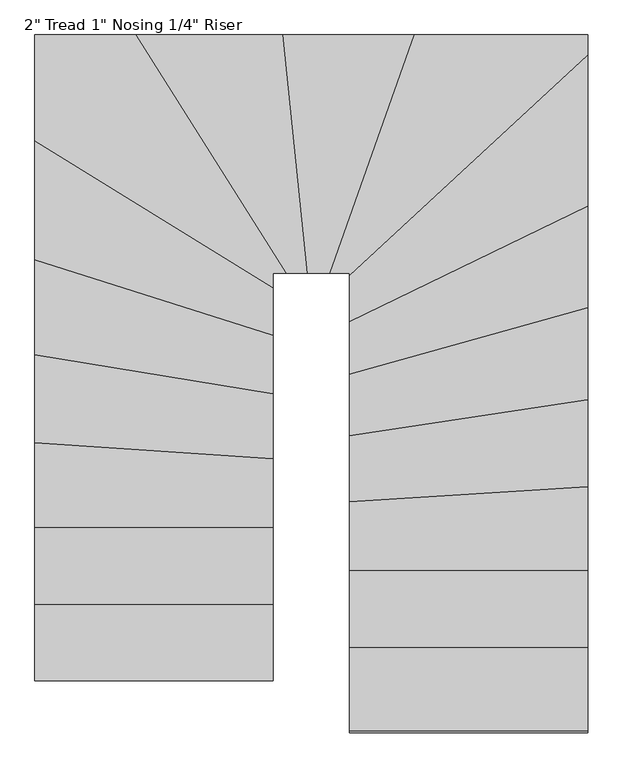
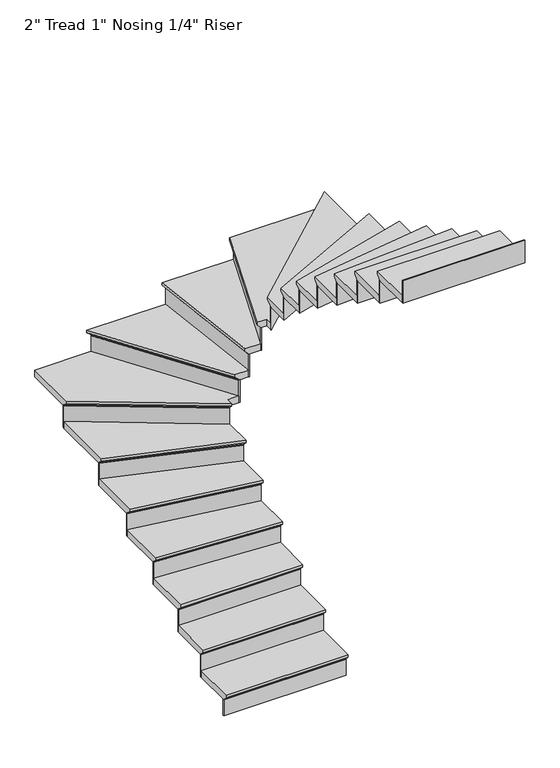
"""IFC4 building model written with IfcOpenShell, lengths in millimetres: stair flight geometry."""

from ifc_helpers import new_model, si_unit, origin, place, context, project, spatial, faceted_brep, source, transform, mapped, element, save


def stair_flight_58ce975e(model_context):
    return source(origin(), model_context, "Body", "Brep", [
        faceted_brep([(2891.8207007, 3072.6312797, 150.2833333), (2891.8207007, 3072.6312797, 169.3333333), (2022.930644, 3072.6312797, 169.3333333), (2022.930644, 3072.6312797, 150.2833333), (2891.8207007, 3098.0312797, 124.8833333), (2022.930644, 3098.0312797, 124.8833333), (2891.8207007, 3377.4312797, 169.3333333), (2022.930644, 3377.4312797, 169.3333333), (2022.930644, 3098.0312797, 118.5333333), (2022.930644, 3377.4312797, 118.5333333), (2891.8207007, 3377.4312797, 118.5333333), (2891.8207007, 3098.0312797, 118.5333333)], [[[0, 1, 2, 3]], [[4, 0, 3, 5]], [[2, 1, 6, 7]], [[8, 9, 10, 11]], [[2, 7, 9, 8, 5, 3]], [[8, 11, 4, 5]], [[6, 1, 0, 4, 11, 10]], [[7, 6, 10, 9]]]),
        faceted_brep([(2891.8207007, 3098.0312797, 118.5333333), (2891.8207007, 3098.0312797, 0.0), (2891.8207007, 3104.3812797, 0.0), (2891.8207007, 3104.3812797, 118.5333333), (2022.930644, 3098.0312797, 118.5333333), (2022.930644, 3104.3812797, 118.5333333), (2022.930644, 3104.3812797, 0.0), (2022.930644, 3098.0312797, 0.0)], [[[0, 1, 2, 3]], [[4, 5, 6, 7]], [[1, 0, 4, 7]], [[2, 1, 7, 6]], [[3, 2, 6, 5]], [[0, 3, 5, 4]]]),
        faceted_brep([(2891.8207007, 3377.4312797, 287.8666667), (2891.8207007, 3377.4312797, 118.5333333), (2891.8207007, 3383.7812797, 118.5333333), (2891.8207007, 3383.7812797, 287.8666667), (2022.930644, 3377.4312797, 287.8666667), (2022.930644, 3383.7812797, 287.8666667), (2022.930644, 3383.7812797, 118.5333333), (2022.930644, 3377.4312797, 118.5333333)], [[[0, 1, 2, 3]], [[4, 5, 6, 7]], [[1, 0, 4, 7]], [[2, 1, 7, 6]], [[3, 2, 6, 5]], [[0, 3, 5, 4]]]),
        faceted_brep([(2022.930644, 3352.0312797, 338.6666667), (2891.8207007, 3352.0312797, 338.6666667), (2891.8207007, 3656.8312797, 338.6666667), (2022.930644, 3656.8312797, 338.6666667), (2022.930644, 3377.4312797, 287.8666667), (2022.930644, 3656.8312797, 287.8666667), (2891.8207007, 3656.8312797, 287.8666667), (2891.8207007, 3377.4312797, 287.8666667), (2022.930644, 3377.4312797, 294.2166667), (2022.930644, 3352.0312797, 319.6166667), (2891.8207007, 3377.4312797, 294.2166667), (2891.8207007, 3352.0312797, 319.6166667)], [[[0, 1, 2, 3]], [[4, 5, 6, 7]], [[0, 3, 5, 4, 8, 9]], [[4, 7, 10, 8]], [[2, 1, 11, 10, 7, 6]], [[3, 2, 6, 5]], [[11, 1, 0, 9]], [[10, 11, 9, 8]]]),
        faceted_brep([(2891.8207007, 3656.8312797, 457.2), (2891.8207007, 3656.8312797, 287.8666667), (2891.8207007, 3663.1812797, 287.8666667), (2891.8207007, 3663.1812797, 457.2), (2022.930644, 3656.8312797, 457.2), (2022.930644, 3663.1812797, 457.2), (2022.930644, 3663.1812797, 287.8666667), (2022.930644, 3656.8312797, 287.8666667)], [[[0, 1, 2, 3]], [[4, 5, 6, 7]], [[1, 0, 4, 7]], [[2, 1, 7, 6]], [[3, 2, 6, 5]], [[0, 3, 5, 4]]]),
        faceted_brep([(2022.930644, 3631.4312797, 508.0), (2891.8207007, 3631.4312797, 508.0), (2891.8207007, 3907.4289831, 508.0), (2022.930644, 3965.1455269, 508.0), (2022.930644, 3656.8312797, 457.2), (2022.930644, 3965.1455269, 457.2), (2891.8207007, 3907.4289831, 457.2), (2891.8207007, 3656.8312797, 457.2), (2022.930644, 3656.8312797, 463.55), (2022.930644, 3631.4312797, 488.95), (2891.8207007, 3656.8312797, 463.55), (2891.8207007, 3631.4312797, 488.95)], [[[0, 1, 2, 3]], [[4, 5, 6, 7]], [[0, 3, 5, 4, 8, 9]], [[4, 7, 10, 8]], [[2, 1, 11, 10, 7, 6]], [[3, 2, 6, 5]], [[11, 1, 0, 9]], [[10, 11, 9, 8]]]),
        faceted_brep([(2891.8207007, 3907.4289831, 626.5333333), (2891.8207007, 3907.4289831, 457.2), (2891.8207007, 3913.7929769, 457.2), (2891.8207007, 3913.7929769, 626.5333333), (2022.930644, 3965.1455269, 626.5333333), (2022.930644, 3971.5095207, 626.5333333), (2022.930644, 3971.5095207, 457.2), (2022.930644, 3965.1455269, 457.2)], [[[0, 1, 2, 3]], [[4, 5, 6, 7]], [[1, 0, 4, 7]], [[2, 1, 7, 6]], [[3, 2, 6, 5]], [[0, 3, 5, 4]]]),
        faceted_brep([(2022.930644, 3939.6895516, 677.3333333), (2891.8207007, 3881.9730078, 677.3333333), (2891.8207007, 4145.020606, 677.3333333), (2022.930644, 4286.9148786, 677.3333333), (2022.930644, 3965.1455269, 626.5333333), (2022.930644, 4286.9148786, 626.5333333), (2891.8207007, 4145.020606, 626.5333333), (2891.8207007, 3907.4289831, 626.5333333), (2022.930644, 3965.1455269, 632.8833333), (2022.930644, 3939.6895516, 658.2833333), (2891.8207007, 3907.4289831, 632.8833333), (2891.8207007, 3881.9730078, 658.2833333)], [[[0, 1, 2, 3]], [[4, 5, 6, 7]], [[0, 3, 5, 4, 8, 9]], [[4, 7, 10, 8]], [[2, 1, 11, 10, 7, 6]], [[3, 2, 6, 5]], [[11, 1, 0, 9]], [[10, 11, 9, 8]]]),
        faceted_brep([(2891.8207007, 4145.020606, 795.8666667), (2891.8207007, 4145.020606, 626.5333333), (2891.8207007, 4151.4547217, 626.5333333), (2891.8207007, 4151.4547217, 795.8666667), (2022.930644, 4286.9148786, 795.8666667), (2022.930644, 4293.3489943, 795.8666667), (2022.930644, 4293.3489943, 626.5333333), (2022.930644, 4286.9148786, 626.5333333)], [[[0, 1, 2, 3]], [[4, 5, 6, 7]], [[1, 0, 4, 7]], [[2, 1, 7, 6]], [[3, 2, 6, 5]], [[0, 3, 5, 4]]]),
        faceted_brep([(2022.930644, 4261.178416, 846.6666667), (2891.8207007, 4119.2841434, 846.6666667), (2891.8207007, 4358.2118283, 846.6666667), (2022.930644, 4634.3545236, 846.6666667), (2022.930644, 4286.9148786, 795.8666667), (2022.930644, 4634.3545236, 795.8666667), (2891.8207007, 4358.2118283, 795.8666667), (2891.8207007, 4145.020606, 795.8666667), (2022.930644, 4286.9148786, 802.2166667), (2022.930644, 4261.178416, 827.6166667), (2891.8207007, 4145.020606, 802.2166667), (2891.8207007, 4119.2841434, 827.6166667)], [[[0, 1, 2, 3]], [[4, 5, 6, 7]], [[0, 3, 5, 4, 8, 9]], [[4, 7, 10, 8]], [[2, 1, 11, 10, 7, 6]], [[3, 2, 6, 5]], [[11, 1, 0, 9]], [[10, 11, 9, 8]]]),
        faceted_brep([(2891.8207007, 4358.2118283, 965.2), (2891.8207007, 4358.2118283, 795.8666667), (2891.8207007, 4364.8748024, 795.8666667), (2891.8207007, 4364.8748024, 965.2), (2022.930644, 4634.3545236, 965.2), (2022.930644, 4641.0174977, 965.2), (2022.930644, 4641.0174977, 795.8666667), (2022.930644, 4634.3545236, 795.8666667)], [[[0, 1, 2, 3]], [[4, 5, 6, 7]], [[1, 0, 4, 7]], [[2, 1, 7, 6]], [[3, 2, 6, 5]], [[0, 3, 5, 4]]]),
        faceted_brep([(2022.930644, 4607.7026274, 1016.0), (2891.8207007, 4331.559932, 1016.0), (2891.8207007, 4534.5950864, 1016.0), (2022.930644, 5069.5207631, 1016.0), (2022.930644, 4634.3545236, 965.2), (2022.930644, 5069.5207631, 965.2), (2891.8207007, 4534.5950864, 965.2), (2891.8207007, 4358.2118283, 965.2), (2022.930644, 4634.3545236, 971.55), (2022.930644, 4607.7026274, 996.95), (2891.8207007, 4358.2118283, 971.55), (2891.8207007, 4331.559932, 996.95)], [[[0, 1, 2, 3]], [[4, 5, 6, 7]], [[0, 3, 5, 4, 8, 9]], [[4, 7, 10, 8]], [[2, 1, 11, 10, 7, 6]], [[3, 2, 6, 5]], [[11, 1, 0, 9]], [[10, 11, 9, 8]]]),
        faceted_brep([(2891.8207007, 4534.5950864, 1134.5333333), (2891.8207007, 4534.5950864, 965.2), (2891.8207007, 4542.0519866, 965.2), (2891.8207007, 4542.0519866, 1134.5333333), (2022.930644, 5069.5207631, 1134.5333333), (2022.930644, 5076.9776634, 1134.5333333), (2022.930644, 5076.9776634, 965.2), (2022.930644, 5069.5207631, 965.2)], [[[0, 1, 2, 3]], [[4, 5, 6, 7]], [[1, 0, 4, 7]], [[2, 1, 7, 6]], [[3, 2, 6, 5]], [[0, 3, 5, 4]]]),
        faceted_brep([(2422.615416, 5425.8753925, 1185.3333333), (2022.930644, 5425.8753925, 1185.3333333), (2022.930644, 5039.693162, 1185.3333333), (2891.8207007, 4504.7674852, 1185.3333333), (2891.8207007, 4556.9853358, 1185.3333333), (2971.434334, 4556.9853358, 1185.3333333), (2022.930644, 5425.8753925, 1134.5333333), (2422.615416, 5425.8753925, 1134.5333333), (2971.434334, 4556.9853358, 1134.5333333), (2891.8207007, 4556.9853358, 1134.5333333), (2891.8207007, 4534.5950864, 1134.5333333), (2022.930644, 5069.5207631, 1134.5333333), (2022.930644, 5069.5207631, 1140.8833333), (2022.930644, 5039.693162, 1166.2833333), (2891.8207007, 4534.5950864, 1140.8833333), (2891.8207007, 4504.7674852, 1166.2833333)], [[[0, 1, 2, 3, 4, 5]], [[6, 7, 8, 9, 10, 11]], [[1, 0, 7, 6]], [[2, 1, 6, 11, 12, 13]], [[11, 10, 14, 12]], [[4, 3, 15, 14, 10, 9]], [[5, 4, 9, 8]], [[0, 5, 8, 7]], [[15, 3, 2, 13]], [[14, 15, 13, 12]]]),
        faceted_brep([(2971.434334, 4556.9853358, 1303.8666667), (2971.434334, 4556.9853358, 1134.5333333), (2978.944962, 4556.9853358, 1134.5333333), (2978.944962, 4556.9853358, 1303.8666667), (2422.615416, 5425.8753925, 1303.8666667), (2430.1260439, 5425.8753925, 1303.8666667), (2430.1260439, 5425.8753925, 1134.5333333), (2422.615416, 5425.8753925, 1134.5333333)], [[[0, 1, 2, 3]], [[4, 5, 6, 7]], [[1, 0, 4, 7]], [[2, 1, 7, 6]], [[3, 2, 6, 5]], [[0, 3, 5, 4]]]),
        faceted_brep([(2392.5729041, 5425.8753925, 1354.6666667), (2941.3918221, 4556.9853358, 1354.6666667), (3041.9537098, 4556.9853358, 1354.6666667), (2952.7958702, 5425.8753925, 1354.6666667), (2422.615416, 5425.8753925, 1303.8666667), (2952.7958702, 5425.8753925, 1303.8666667), (3041.9537098, 4556.9853358, 1303.8666667), (2971.434334, 4556.9853358, 1303.8666667), (2422.615416, 5425.8753925, 1310.2166667), (2392.5729041, 5425.8753925, 1335.6166667), (2971.434334, 4556.9853358, 1310.2166667), (2941.3918221, 4556.9853358, 1335.6166667)], [[[0, 1, 2, 3]], [[4, 5, 6, 7]], [[0, 3, 5, 4, 8, 9]], [[4, 7, 10, 8]], [[3, 2, 6, 5]], [[11, 1, 0, 9]], [[10, 11, 9, 8]], [[2, 1, 11, 10, 7, 6]]]),
        faceted_brep([(3041.9537098, 4556.9853358, 1473.2), (3041.9537098, 4556.9853358, 1303.8666667), (3048.337052, 4556.9853358, 1303.8666667), (3048.337052, 4556.9853358, 1473.2), (2952.7958702, 5425.8753925, 1473.2), (2959.1792124, 5425.8753925, 1473.2), (2959.1792124, 5425.8753925, 1303.8666667), (2952.7958702, 5425.8753925, 1303.8666667)], [[[0, 1, 2, 3]], [[4, 5, 6, 7]], [[1, 0, 4, 7]], [[2, 1, 7, 6]], [[3, 2, 6, 5]], [[0, 3, 5, 4]]]),
        faceted_brep([(2927.2625013, 5425.8753925, 1524.0), (3016.420341, 4556.9853358, 1524.0), (3126.725754, 4556.9853358, 1524.0), (3434.7136561, 5425.8753925, 1524.0), (2952.7958702, 5425.8753925, 1473.2), (3434.7136561, 5425.8753925, 1473.2), (3126.725754, 4556.9853358, 1473.2), (3041.9537098, 4556.9853358, 1473.2), (2952.7958702, 5425.8753925, 1479.55), (2927.2625013, 5425.8753925, 1504.95), (3041.9537098, 4556.9853358, 1479.55), (3016.420341, 4556.9853358, 1504.95)], [[[0, 1, 2, 3]], [[4, 5, 6, 7]], [[0, 3, 5, 4, 8, 9]], [[4, 7, 10, 8]], [[2, 1, 11, 10, 7, 6]], [[3, 2, 6, 5]], [[11, 1, 0, 9]], [[10, 11, 9, 8]]]),
        faceted_brep([(3126.725754, 4556.9853358, 1642.5333333), (3126.725754, 4556.9853358, 1473.2), (3133.46287, 4556.9853358, 1473.2), (3133.46287, 4556.9853358, 1642.5333333), (3434.7136561, 5425.8753925, 1642.5333333), (3441.4507721, 5425.8753925, 1642.5333333), (3441.4507721, 5425.8753925, 1473.2), (3434.7136561, 5425.8753925, 1473.2)], [[[0, 1, 2, 3]], [[4, 5, 6, 7]], [[1, 0, 4, 7]], [[2, 1, 7, 6]], [[3, 2, 6, 5]], [[0, 3, 5, 4]]]),
        faceted_brep([(4040.1107574, 5316.6559739, 1693.3333333), (4040.1107574, 5425.8753925, 1693.3333333), (3407.7651919, 5425.8753925, 1693.3333333), (3099.7772899, 4556.9853358, 1693.3333333), (3171.2207007, 4556.9853358, 1693.3333333), (3171.2207007, 4513.460321, 1693.3333333), (4040.1107574, 5425.8753925, 1642.5333333), (4040.1107574, 5316.6559739, 1642.5333333), (3171.2207007, 4513.460321, 1642.5333333), (3171.2207007, 4556.9853358, 1642.5333333), (3126.725754, 4556.9853358, 1642.5333333), (3434.7136561, 5425.8753925, 1642.5333333), (3126.725754, 4556.9853358, 1648.8833333), (3434.7136561, 5425.8753925, 1648.8833333), (3099.7772899, 4556.9853358, 1674.2833333), (3407.7651919, 5425.8753925, 1674.2833333)], [[[0, 1, 2, 3, 4, 5]], [[6, 7, 8, 9, 10, 11]], [[1, 0, 7, 6]], [[11, 10, 12, 13]], [[4, 3, 14, 12, 10, 9]], [[5, 4, 9, 8]], [[0, 5, 8, 7]], [[14, 3, 2, 15]], [[12, 14, 15, 13]], [[2, 1, 6, 11, 13, 15]]]),
        faceted_brep([(3171.2207007, 4513.460321, 1811.8666667), (3171.2207007, 4513.460321, 1642.5333333), (3171.2207007, 4504.8128847, 1642.5333333), (3171.2207007, 4504.8128847, 1811.8666667), (4040.1107574, 5316.6559739, 1811.8666667), (4040.1107574, 5308.0085377, 1811.8666667), (4040.1107574, 5308.0085377, 1642.5333333), (4040.1107574, 5316.6559739, 1642.5333333)], [[[0, 1, 2, 3]], [[4, 5, 6, 7]], [[1, 0, 4, 7]], [[2, 1, 7, 6]], [[3, 2, 6, 5]], [[0, 3, 5, 4]]]),
        faceted_brep([(4040.1107574, 5351.245719, 1862.6666667), (3171.2207007, 4548.050066, 1862.6666667), (3171.2207007, 4351.7726611, 1862.6666667), (4040.1107574, 4773.173215, 1862.6666667), (4040.1107574, 5316.6559739, 1811.8666667), (4040.1107574, 4773.173215, 1811.8666667), (3171.2207007, 4351.7726611, 1811.8666667), (3171.2207007, 4513.460321, 1811.8666667), (4040.1107574, 5316.6559739, 1818.2166667), (4040.1107574, 5351.245719, 1843.6166667), (3171.2207007, 4513.460321, 1818.2166667), (3171.2207007, 4548.050066, 1843.6166667)], [[[0, 1, 2, 3]], [[4, 5, 6, 7]], [[0, 3, 5, 4, 8, 9]], [[4, 7, 10, 8]], [[2, 1, 11, 10, 7, 6]], [[3, 2, 6, 5]], [[11, 1, 0, 9]], [[10, 11, 9, 8]]]),
        faceted_brep([(3171.2207007, 4351.7726611, 1981.2), (3171.2207007, 4351.7726611, 1811.8666667), (3171.2207007, 4344.7152636, 1811.8666667), (3171.2207007, 4344.7152636, 1981.2), (4040.1107574, 4773.173215, 1981.2), (4040.1107574, 4766.1158175, 1981.2), (4040.1107574, 4766.1158175, 1811.8666667), (4040.1107574, 4773.173215, 1811.8666667)], [[[0, 1, 2, 3]], [[4, 5, 6, 7]], [[1, 0, 4, 7]], [[2, 1, 7, 6]], [[3, 2, 6, 5]], [[0, 3, 5, 4]]]),
        faceted_brep([(4040.1107574, 4801.4028049, 2032.0), (3171.2207007, 4380.002251, 2032.0), (3171.2207007, 4163.4811416, 2032.0), (4040.1107574, 4405.175707, 2032.0), (4040.1107574, 4773.173215, 1981.2), (4040.1107574, 4405.175707, 1981.2), (3171.2207007, 4163.4811416, 1981.2), (3171.2207007, 4351.7726611, 1981.2), (4040.1107574, 4773.173215, 1987.55), (4040.1107574, 4801.4028049, 2012.95), (3171.2207007, 4351.7726611, 1987.55), (3171.2207007, 4380.002251, 2012.95)], [[[0, 1, 2, 3]], [[4, 5, 6, 7]], [[0, 3, 5, 4, 8, 9]], [[4, 7, 10, 8]], [[2, 1, 11, 10, 7, 6]], [[3, 2, 6, 5]], [[11, 1, 0, 9]], [[10, 11, 9, 8]]]),
        faceted_brep([(3171.2207007, 4163.4811416, 2150.5333333), (3171.2207007, 4163.4811416, 1981.2), (3171.2207007, 4156.8900508, 1981.2), (3171.2207007, 4156.8900508, 2150.5333333), (4040.1107574, 4405.175707, 2150.5333333), (4040.1107574, 4398.5846162, 2150.5333333), (4040.1107574, 4398.5846162, 1981.2), (4040.1107574, 4405.175707, 1981.2)], [[[0, 1, 2, 3]], [[4, 5, 6, 7]], [[1, 0, 4, 7]], [[2, 1, 7, 6]], [[3, 2, 6, 5]], [[0, 3, 5, 4]]]),
        faceted_brep([(4040.1107574, 4431.5400703, 2201.3333333), (3171.2207007, 4189.8455049, 2201.3333333), (3171.2207007, 3940.3652675, 2201.3333333), (4040.1107574, 4070.8506687, 2201.3333333), (4040.1107574, 4405.175707, 2150.5333333), (4040.1107574, 4070.8506687, 2150.5333333), (3171.2207007, 3940.3652675, 2150.5333333), (3171.2207007, 4163.4811416, 2150.5333333), (4040.1107574, 4405.175707, 2156.8833333), (4040.1107574, 4431.5400703, 2182.2833333), (3171.2207007, 4163.4811416, 2156.8833333), (3171.2207007, 4189.8455049, 2182.2833333)], [[[0, 1, 2, 3]], [[4, 5, 6, 7]], [[0, 3, 5, 4, 8, 9]], [[4, 7, 10, 8]], [[2, 1, 11, 10, 7, 6]], [[3, 2, 6, 5]], [[11, 1, 0, 9]], [[10, 11, 9, 8]]]),
        faceted_brep([(3171.2207007, 3940.3652675, 2319.8666667), (3171.2207007, 3940.3652675, 2150.5333333), (3171.2207007, 3933.9440626, 2150.5333333), (3171.2207007, 3933.9440626, 2319.8666667), (4040.1107574, 4070.8506687, 2319.8666667), (4040.1107574, 4064.4294638, 2319.8666667), (4040.1107574, 4064.4294638, 2150.5333333), (4040.1107574, 4070.8506687, 2150.5333333)], [[[0, 1, 2, 3]], [[4, 5, 6, 7]], [[1, 0, 4, 7]], [[2, 1, 7, 6]], [[3, 2, 6, 5]], [[0, 3, 5, 4]]]),
        faceted_brep([(4040.1107574, 4096.5354882, 2370.6666667), (3171.2207007, 3966.050087, 2370.6666667), (3171.2207007, 3699.03363, 2370.6666667), (4040.1107574, 3753.8509483, 2370.6666667), (4040.1107574, 4070.8506687, 2319.8666667), (4040.1107574, 3753.8509483, 2319.8666667), (3171.2207007, 3699.03363, 2319.8666667), (3171.2207007, 3940.3652675, 2319.8666667), (4040.1107574, 4070.8506687, 2326.2166667), (4040.1107574, 4096.5354882, 2351.6166667), (3171.2207007, 3940.3652675, 2326.2166667), (3171.2207007, 3966.050087, 2351.6166667)], [[[0, 1, 2, 3]], [[4, 5, 6, 7]], [[0, 3, 5, 4, 8, 9]], [[4, 7, 10, 8]], [[2, 1, 11, 10, 7, 6]], [[3, 2, 6, 5]], [[11, 1, 0, 9]], [[10, 11, 9, 8]]]),
        faceted_brep([(3171.2207007, 3699.03363, 2489.2), (3171.2207007, 3699.03363, 2319.8666667), (3171.2207007, 3692.6710054, 2319.8666667), (3171.2207007, 3692.6710054, 2489.2), (4040.1107574, 3753.8509483, 2489.2), (4040.1107574, 3747.4883236, 2489.2), (4040.1107574, 3747.4883236, 2319.8666667), (4040.1107574, 3753.8509483, 2319.8666667)], [[[0, 1, 2, 3]], [[4, 5, 6, 7]], [[1, 0, 4, 7]], [[2, 1, 7, 6]], [[3, 2, 6, 5]], [[0, 3, 5, 4]]]),
        faceted_brep([(4040.1107574, 3779.3014467, 2540.0), (3171.2207007, 3724.4841285, 2540.0), (3171.2207007, 3447.0927876, 2540.0), (4040.1107574, 3447.0927876, 2540.0), (4040.1107574, 3753.8509483, 2489.2), (4040.1107574, 3447.0927876, 2489.2), (3171.2207007, 3447.0927876, 2489.2), (3171.2207007, 3699.03363, 2489.2), (4040.1107574, 3753.8509483, 2495.55), (4040.1107574, 3779.3014467, 2520.95), (3171.2207007, 3699.03363, 2495.55), (3171.2207007, 3724.4841285, 2520.95)], [[[0, 1, 2, 3]], [[4, 5, 6, 7]], [[0, 3, 5, 4, 8, 9]], [[4, 7, 10, 8]], [[2, 1, 11, 10, 7, 6]], [[3, 2, 6, 5]], [[11, 1, 0, 9]], [[10, 11, 9, 8]]]),
        faceted_brep([(3171.2207007, 3447.0927876, 2658.5333333), (3171.2207007, 3447.0927876, 2489.2), (3171.2207007, 3440.7427876, 2489.2), (3171.2207007, 3440.7427876, 2658.5333333), (4040.1107574, 3447.0927876, 2658.5333333), (4040.1107574, 3440.7427876, 2658.5333333), (4040.1107574, 3440.7427876, 2489.2), (4040.1107574, 3447.0927876, 2489.2)], [[[0, 1, 2, 3]], [[4, 5, 6, 7]], [[1, 0, 4, 7]], [[2, 1, 7, 6]], [[3, 2, 6, 5]], [[0, 3, 5, 4]]]),
        faceted_brep([(4040.1107574, 3472.4927876, 2709.3333333), (3171.2207007, 3472.4927876, 2709.3333333), (3171.2207007, 3167.6927876, 2709.3333333), (4040.1107574, 3167.6927876, 2709.3333333), (4040.1107574, 3447.0927876, 2658.5333333), (4040.1107574, 3167.6927876, 2658.5333333), (3171.2207007, 3167.6927876, 2658.5333333), (3171.2207007, 3447.0927876, 2658.5333333), (4040.1107574, 3447.0927876, 2664.8833333), (4040.1107574, 3472.4927876, 2690.2833333), (3171.2207007, 3447.0927876, 2664.8833333), (3171.2207007, 3472.4927876, 2690.2833333)], [[[0, 1, 2, 3]], [[4, 5, 6, 7]], [[0, 3, 5, 4, 8, 9]], [[4, 7, 10, 8]], [[2, 1, 11, 10, 7, 6]], [[3, 2, 6, 5]], [[11, 1, 0, 9]], [[10, 11, 9, 8]]]),
        faceted_brep([(3171.2207007, 3167.6927876, 2827.8666667), (3171.2207007, 3167.6927876, 2658.5333333), (3171.2207007, 3161.3427876, 2658.5333333), (3171.2207007, 3161.3427876, 2827.8666667), (4040.1107574, 3167.6927876, 2827.8666667), (4040.1107574, 3161.3427876, 2827.8666667), (4040.1107574, 3161.3427876, 2658.5333333), (4040.1107574, 3167.6927876, 2658.5333333)], [[[0, 1, 2, 3]], [[4, 5, 6, 7]], [[1, 0, 4, 7]], [[2, 1, 7, 6]], [[3, 2, 6, 5]], [[0, 3, 5, 4]]]),
        faceted_brep([(3171.2207007, 2888.2927876, 2997.2), (3171.2207007, 2888.2927876, 2827.8666667), (3171.2207007, 2881.9427876, 2827.8666667), (3171.2207007, 2881.9427876, 2997.2), (4040.1107574, 2888.2927876, 2997.2), (4040.1107574, 2881.9427876, 2997.2), (4040.1107574, 2881.9427876, 2827.8666667), (4040.1107574, 2888.2927876, 2827.8666667)], [[[0, 1, 2, 3]], [[4, 5, 6, 7]], [[1, 0, 4, 7]], [[2, 1, 7, 6]], [[3, 2, 6, 5]], [[0, 3, 5, 4]]]),
        faceted_brep([(4040.1107574, 3193.0927876, 2878.6666667), (3171.2207007, 3193.0927876, 2878.6666667), (3171.2207007, 2888.2927876, 2878.6666667), (4040.1107574, 2888.2927876, 2878.6666667), (4040.1107574, 3167.6927876, 2827.8666667), (4040.1107574, 2888.2927876, 2827.8666667), (3171.2207007, 2888.2927876, 2827.8666667), (3171.2207007, 3167.6927876, 2827.8666667), (4040.1107574, 3167.6927876, 2834.2166667), (4040.1107574, 3193.0927876, 2859.6166667), (3171.2207007, 3167.6927876, 2834.2166667), (3171.2207007, 3193.0927876, 2859.6166667)], [[[0, 1, 2, 3]], [[4, 5, 6, 7]], [[0, 3, 5, 4, 8, 9]], [[4, 7, 10, 8]], [[2, 1, 11, 10, 7, 6]], [[3, 2, 6, 5]], [[11, 1, 0, 9]], [[10, 11, 9, 8]]]),
    ])


if __name__ == "__main__":
    model = new_model("IFC4")
    model_context = context("Model", 3, world=origin())
    ifc_project = project(units=[si_unit("LENGTHUNIT", "METRE", prefix="MILLI")], contexts=[model_context])
    site = spatial("IfcSite", under=ifc_project)
    building = spatial("IfcBuilding", under=site)
    placement = place(None, origin())
    stair_flight_shape = stair_flight_58ce975e(model_context)
    element("IfcStairFlight", 1, ObjectType="2\" Tread 1\" Nosing 1/4\" Riser", at=placement, inside=building, context=model_context, shape_type="MappedRepresentation", body=[
        mapped(stair_flight_shape, transform((0.0, 0.0, 0.0), x_axis=(1.0, 0.0, 0.0), y_axis=(0.0, 1.0, 0.0), z_axis=(0.0, 0.0, 1.0))),
    ])
    save(model, "model.ifc")
